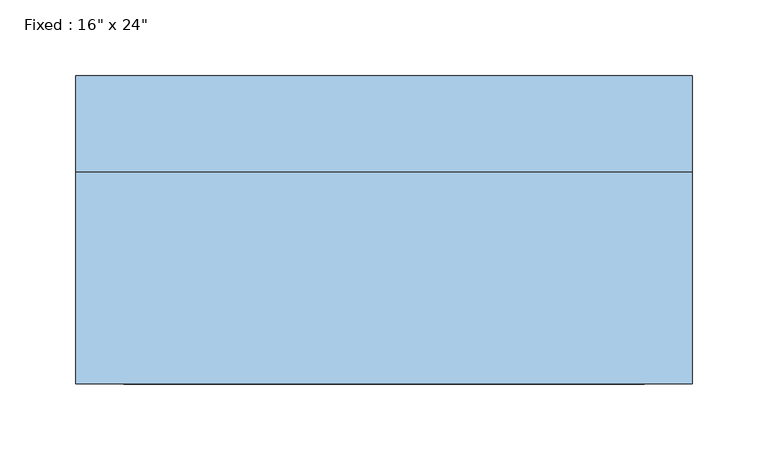
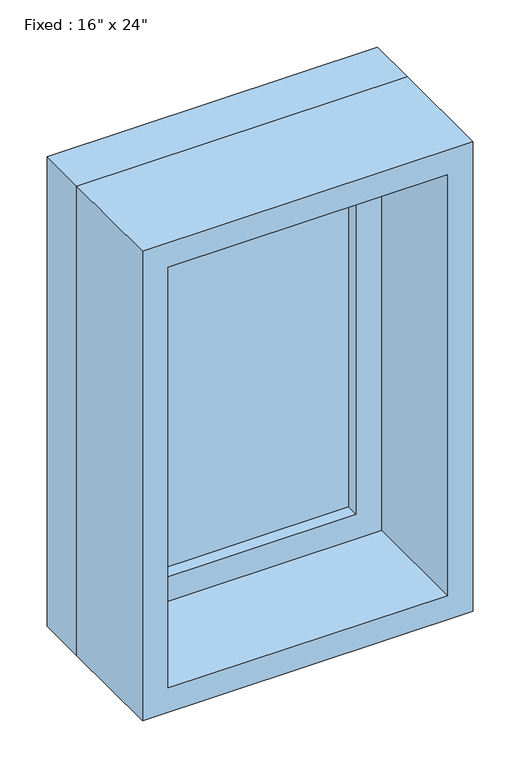
"""IFC4 building model written with IfcOpenShell, lengths in millimetres: window geometry."""

from ifc_helpers import new_model, si_unit, frame, origin, place, context, project, spatial, polyline, outline, extrude, source, transform, mapped, element, save


def window_085f26e1(model_context):
    return source(origin(), model_context, "Body", "SweptSolid", [
        extrude(outline(polyline([(101.6, 53.975), (-177.8, 53.975), (-177.8, 66.675), (101.6, 66.675), (101.6, 53.975)])), frame((0.0, 0.0, 977.9), z_axis=(0.0, 0.0, 1.0), x_axis=(1.0, 0.0, 0.0)), (0.0, 0.0, 1.0), 482.6),
        extrude(outline(polyline([(1504.95, -222.25), (933.45, -222.25), (933.45, 146.05), (1504.95, 146.05), (1504.95, -222.25)]), holes=[polyline([(1460.5, -177.8), (1460.5, 101.6), (977.9, 101.6), (977.9, -177.8), (1460.5, -177.8)])]), frame((0.0, 38.1, 0.0), z_axis=(0.0, 1.0, 0.0), x_axis=(0.0, 0.0, 1.0)), (0.0, 0.0, 1.0), 44.45),
        extrude(outline(polyline([(1524.0, -241.3), (914.4, -241.3), (914.4, 165.1), (1524.0, 165.1), (1524.0, -241.3)]), holes=[polyline([(1492.25, -209.55), (1492.25, 133.35), (946.15, 133.35), (946.15, -209.55), (1492.25, -209.55)])]), frame((0.0, -101.6, 0.0), z_axis=(0.0, 1.0, 0.0), x_axis=(0.0, 0.0, 1.0)), (0.0, 0.0, 1.0), 139.7),
        extrude(outline(polyline([(1524.0, 165.1), (1524.0, -241.3), (914.4, -241.3), (914.4, 165.1), (1524.0, 165.1)]), holes=[polyline([(1504.95, 146.05), (933.45, 146.05), (933.45, -222.25), (1504.95, -222.25), (1504.95, 146.05)])]), frame((0.0, 38.1, 0.0), z_axis=(0.0, 1.0, 0.0), x_axis=(0.0, 0.0, 1.0)), (0.0, 0.0, 1.0), 63.5),
    ])


if __name__ == "__main__":
    model = new_model("IFC4")
    model_context = context("Model", 3, world=origin())
    ifc_project = project(units=[si_unit("LENGTHUNIT", "METRE", prefix="MILLI")], contexts=[model_context])
    site = spatial("IfcSite", under=ifc_project)
    building = spatial("IfcBuilding", under=site)
    placement = place(None, origin())
    window_shape = window_085f26e1(model_context)
    element("IfcWindow", 1, ObjectType="Fixed : 16\" x 24\"", at=placement, inside=building, context=model_context, shape_type="MappedRepresentation", body=[
        mapped(window_shape, transform((0.0, 0.0, 0.0), x_axis=(1.0, 0.0, 0.0), y_axis=(0.0, 1.0, 0.0), z_axis=(0.0, 0.0, 1.0))),
    ])
    save(model, "model.ifc")

# Revit data of these elements
# Type "Fixed : 16\" x 24\""
#   Type Mark = "4"
#   Construction Type Id = "GSP4R"
#   Assembly Code = "B2020100"
#   Analytic Construction = "1/8 in Pilkington single glazing"
#   Visual Light Transmittance = 0.9
#   Solar Heat Gain Coefficient = 0.78
#   Heat Transfer Coefficient (U) = 0.6496 BTU/(h·ft²·°F)
#   Height = 2' - 0"
#   Default Sill Height = 3' - 0"
#   Width = 1' - 4"
#   Window Inset = 0' - 0 3/4"
#   Define Thermal Properties by = 1
#   Define Thermal Properties by = 1
#   Glass Pane Material = Glass
#   Sash Material = Sash
#   Wall Closure = (empty or 0)
# Element 1 (IfcWindow, "Fixed : 16\" x 24\"")
#   Materials on its faces: "Sash", "Glass"
# Materials
#   "Glass": class "Glass", colour RGB 0 128 192, transparency 0.75, Description = "Soda Lime Glass", Cost = 0
#   "Sash": class "Wood", colour RGB 224 178 126, transparency 0, Cost = 0
